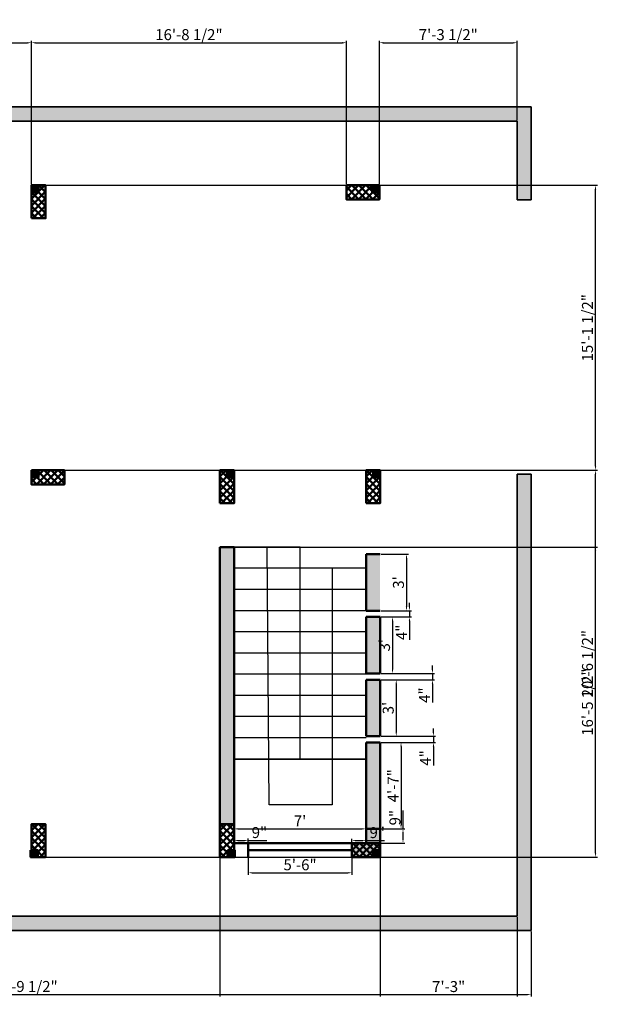
# Model space of a CAD drawing. Units: inches. Extents: x 1749 to 3550, y 1117 to 2383.
# Tile 9 of 15: x 2287 to 2660, y 1756 to 2383. Entities that reach past the tile are written whole.
import ezdxf

# ---------------------------------------------------------------- set-up
doc = ezdxf.new("R2010")
doc.units = ezdxf.units.IN
for name, color, linetype, lineweight in [('A-ANNO-DIMS', 2, 'Continuous', 18), ('A-COLS', 10, 'Continuous', 50), ('A-FLOR-STRS', 53, 'Continuous', 25), ('A-WALL', 7, 'Continuous', 50), ('A-WALL-PATT', 8, 'Continuous', 13), ('C-PROP', 8, 'Continuous', 35)]:
    doc.layers.add(name, color=color, linetype=linetype, lineweight=lineweight)
doc.styles.get("Standard").update_dxf_attribs({"font": 'arial.ttf'})
doc.dimstyles.new('ISO-25', dxfattribs={"dimtxt": 7, "dimasz": 2.5, "dimexe": 1.25, "dimexo": 0.625, "dimtad": 1, "dimdec": 1, "dimlunit": 3, "dimtxsty": 'Standard', "dimcen": 2.5, "dimadec": 0, "dimazin": 0, "dimtfac": 1, "dimtdec": 1, "dimtmove": 0, "dimatfit": 3, "dimfxl": 1, "dimarcsym": 0})

# ---------------------------------------------------------------- blocks, each defined once
blk = doc.blocks.new('*D149')
at = {"layer": 'A-ANNO-DIMS', "color": 0, "lineweight": -2, "ltscale": 0.5, "transparency": 16777216}
for p, q in [((2423.6, 1859.29), (2423.6, 1868.91)), ((2426.1, 1867.66), (2505.1, 1867.66)), ((2507.6, 1859.29), (2507.6, 1868.91))]:
    blk.add_line(p, q, dxfattribs=at)
at = {"layer": 'A-ANNO-DIMS', "color": 0, "ltscale": 0.5, "transparency": 16777216}
for points in [[(2426.1, 1868.08), (2426.1, 1867.24), (2423.6, 1867.66)], [(2505.1, 1868.08), (2505.1, 1867.24), (2507.6, 1867.66)]]:
    blk.add_solid(points, dxfattribs=at)
at = {"layer": 'Defpoints', "color": 0, "ltscale": 0.5, "transparency": 16777216}
for p in [(2507.6, 1867.66), (2423.6, 1858.66), (2507.6, 1858.66)]:
    blk.add_point(p, dxfattribs=at)
at = {"layer": 'A-ANNO-DIMS', "color": 0, "ltscale": 0.5, "transparency": 16777216, "insert": (2465.6, 1871.79), "char_height": 7, "attachment_point": 5}
blk.add_mtext("7'", dxfattribs=at)
blk = doc.blocks.new('*D143')
at = {"layer": 'A-ANNO-DIMS', "color": 0, "lineweight": -2, "ltscale": 0.5, "transparency": 16777216}
for p, q in [((2517.23, 2042.66), (2534.61, 2042.66)), ((2533.36, 2040.16), (2533.36, 2009.16)), ((2517.23, 2006.66), (2534.61, 2006.66))]:
    blk.add_line(p, q, dxfattribs=at)
at = {"layer": 'A-ANNO-DIMS', "color": 0, "ltscale": 0.5, "transparency": 16777216}
for points in [[(2532.94, 2040.16), (2533.78, 2040.16), (2533.36, 2042.66)], [(2532.94, 2009.16), (2533.78, 2009.16), (2533.36, 2006.66)]]:
    blk.add_solid(points, dxfattribs=at)
at = {"layer": 'Defpoints', "color": 0, "ltscale": 0.5, "transparency": 16777216}
for p in [(2516.6, 2042.66), (2516.6, 2006.66), (2533.36, 2006.66)]:
    blk.add_point(p, dxfattribs=at)
at = {"layer": 'A-ANNO-DIMS', "color": 0, "ltscale": 0.5, "transparency": 16777216, "insert": (2529.16, 2024.66), "char_height": 7, "attachment_point": 5, "rotation": 90}
blk.add_mtext("3'", dxfattribs=at)
blk = doc.blocks.new('*D144')
at = {"layer": 'A-ANNO-DIMS', "color": 0, "lineweight": -2, "ltscale": 0.5, "transparency": 16777216}
for p, q in [((2535.25, 2009.16), (2535.25, 2011.66)), ((2517.23, 2006.66), (2536.5, 2006.66)), ((2517.23, 2002.66), (2536.5, 2002.66)), ((2535.25, 2006.66), (2535.25, 2002.66)), ((2535.25, 2000.16), (2535.25, 1988.08))]:
    blk.add_line(p, q, dxfattribs=at)
at = {"layer": 'A-ANNO-DIMS', "color": 0, "ltscale": 0.5, "transparency": 16777216}
for points in [[(2534.83, 2009.16), (2535.66, 2009.16), (2535.25, 2006.66)], [(2534.83, 2000.16), (2535.66, 2000.16), (2535.25, 2002.66)]]:
    blk.add_solid(points, dxfattribs=at)
at = {"layer": 'Defpoints', "color": 0, "ltscale": 0.5, "transparency": 16777216}
for p in [(2516.6, 2006.66), (2516.6, 2002.66), (2535.25, 2002.66)]:
    blk.add_point(p, dxfattribs=at)
at = {"layer": 'A-ANNO-DIMS', "color": 0, "ltscale": 0.5, "transparency": 16777216, "insert": (2531.12, 1992.87), "char_height": 7, "attachment_point": 5, "rotation": 90}
blk.add_mtext('4"', dxfattribs=at)
blk = doc.blocks.new('*D145')
at = {"layer": 'A-ANNO-DIMS', "color": 0, "lineweight": -2, "ltscale": 0.5, "transparency": 16777216}
for p, q in [((2517.23, 2002.66), (2525.75, 2002.66)), ((2524.5, 2000.16), (2524.5, 1969.16)), ((2517.23, 1966.66), (2525.75, 1966.66))]:
    blk.add_line(p, q, dxfattribs=at)
at = {"layer": 'A-ANNO-DIMS', "color": 0, "ltscale": 0.5, "transparency": 16777216}
for points in [[(2524.08, 2000.16), (2524.91, 2000.16), (2524.5, 2002.66)], [(2524.08, 1969.16), (2524.91, 1969.16), (2524.5, 1966.66)]]:
    blk.add_solid(points, dxfattribs=at)
at = {"layer": 'Defpoints', "color": 0, "ltscale": 0.5, "transparency": 16777216}
for p in [(2516.6, 2002.66), (2516.6, 1966.66), (2524.5, 1966.66)]:
    blk.add_point(p, dxfattribs=at)
at = {"layer": 'A-ANNO-DIMS', "color": 0, "ltscale": 0.5, "transparency": 16777216, "insert": (2520.29, 1984.66), "char_height": 7, "attachment_point": 5, "rotation": 90}
blk.add_mtext("3'", dxfattribs=at)
blk = doc.blocks.new('*D146')
at = {"layer": 'A-ANNO-DIMS', "color": 0, "lineweight": -2, "ltscale": 0.5, "transparency": 16777216}
for p, q in [((2549.88, 1969.16), (2549.88, 1971.66)), ((2517.23, 1966.66), (2551.13, 1966.66)), ((2549.88, 1966.66), (2549.88, 1962.66)), ((2517.23, 1962.66), (2551.13, 1962.66)), ((2549.88, 1960.16), (2549.88, 1948.08))]:
    blk.add_line(p, q, dxfattribs=at)
at = {"layer": 'A-ANNO-DIMS', "color": 0, "ltscale": 0.5, "transparency": 16777216}
for points in [[(2549.46, 1969.16), (2550.3, 1969.16), (2549.88, 1966.66)], [(2549.46, 1960.16), (2550.3, 1960.16), (2549.88, 1962.66)]]:
    blk.add_solid(points, dxfattribs=at)
at = {"layer": 'Defpoints', "color": 0, "ltscale": 0.5, "transparency": 16777216}
for p in [(2516.6, 1966.66), (2516.6, 1962.66), (2549.88, 1962.66)]:
    blk.add_point(p, dxfattribs=at)
at = {"layer": 'A-ANNO-DIMS', "color": 0, "ltscale": 0.5, "transparency": 16777216, "insert": (2545.75, 1952.87), "char_height": 7, "attachment_point": 5, "rotation": 90}
blk.add_mtext('4"', dxfattribs=at)
blk = doc.blocks.new('*D147')
at = {"layer": 'A-ANNO-DIMS', "color": 0, "lineweight": -2, "ltscale": 0.5, "transparency": 16777216}
for p, q in [((2517.23, 1962.66), (2528.1, 1962.66)), ((2526.85, 1960.16), (2526.85, 1929.16)), ((2517.23, 1926.66), (2528.1, 1926.66))]:
    blk.add_line(p, q, dxfattribs=at)
at = {"layer": 'A-ANNO-DIMS', "color": 0, "ltscale": 0.5, "transparency": 16777216}
for points in [[(2526.43, 1960.16), (2527.26, 1960.16), (2526.85, 1962.66)], [(2526.43, 1929.16), (2527.26, 1929.16), (2526.85, 1926.66)]]:
    blk.add_solid(points, dxfattribs=at)
at = {"layer": 'Defpoints', "color": 0, "ltscale": 0.5, "transparency": 16777216}
for p in [(2516.6, 1962.66), (2516.6, 1926.66), (2526.85, 1926.66)]:
    blk.add_point(p, dxfattribs=at)
at = {"layer": 'A-ANNO-DIMS', "color": 0, "ltscale": 0.5, "transparency": 16777216, "insert": (2522.64, 1944.66), "char_height": 7, "attachment_point": 5, "rotation": 90}
blk.add_mtext("3'", dxfattribs=at)
blk = doc.blocks.new('*D148')
at = {"layer": 'A-ANNO-DIMS', "color": 0, "lineweight": -2, "ltscale": 0.5, "transparency": 16777216}
for p, q in [((2517.23, 1926.66), (2551.76, 1926.66)), ((2550.51, 1929.16), (2550.51, 1931.66)), ((2550.51, 1926.66), (2550.51, 1922.66)), ((2517.23, 1922.66), (2551.76, 1922.66)), ((2550.51, 1920.16), (2550.51, 1908.08))]:
    blk.add_line(p, q, dxfattribs=at)
at = {"layer": 'A-ANNO-DIMS', "color": 0, "ltscale": 0.5, "transparency": 16777216}
for points in [[(2550.09, 1929.16), (2550.93, 1929.16), (2550.51, 1926.66)], [(2550.09, 1920.16), (2550.93, 1920.16), (2550.51, 1922.66)]]:
    blk.add_solid(points, dxfattribs=at)
at = {"layer": 'Defpoints', "color": 0, "ltscale": 0.5, "transparency": 16777216}
for p in [(2516.6, 1926.66), (2516.6, 1922.66), (2550.51, 1922.66)]:
    blk.add_point(p, dxfattribs=at)
at = {"layer": 'A-ANNO-DIMS', "color": 0, "ltscale": 0.5, "transparency": 16777216, "insert": (2546.38, 1912.87), "char_height": 7, "attachment_point": 5, "rotation": 90}
blk.add_mtext('4"', dxfattribs=at)
blk = doc.blocks.new('*D138')
at = {"layer": 'A-ANNO-DIMS', "color": 0, "lineweight": -2, "ltscale": 0.5, "transparency": 16777216}
for p, q in [((2517.23, 1922.66), (2531.15, 1922.66)), ((2529.9, 1920.16), (2529.9, 1870.16)), ((2517.23, 1867.66), (2531.15, 1867.66))]:
    blk.add_line(p, q, dxfattribs=at)
at = {"layer": 'A-ANNO-DIMS', "color": 0, "ltscale": 0.5, "transparency": 16777216}
for points in [[(2529.48, 1920.16), (2530.31, 1920.16), (2529.9, 1922.66)], [(2529.48, 1870.16), (2530.31, 1870.16), (2529.9, 1867.66)]]:
    blk.add_solid(points, dxfattribs=at)
at = {"layer": 'Defpoints', "color": 0, "ltscale": 0.5, "transparency": 16777216}
for p in [(2516.6, 1922.66), (2516.6, 1867.66), (2529.9, 1867.66)]:
    blk.add_point(p, dxfattribs=at)
at = {"layer": 'A-ANNO-DIMS', "color": 0, "ltscale": 0.5, "transparency": 16777216, "insert": (2525.77, 1895.16), "char_height": 7, "attachment_point": 5, "rotation": 90}
blk.add_mtext('4\'-7"', dxfattribs=at)
blk = doc.blocks.new('*D139')
at = {"layer": 'A-ANNO-DIMS', "color": 0, "lineweight": -2, "ltscale": 0.5, "transparency": 16777216}
for p, q in [((2531.15, 1867.66), (2531.15, 1879.46)), ((2517.23, 1867.66), (2532.4, 1867.66)), ((2531.15, 1861.16), (2531.15, 1865.16)), ((2517.23, 1858.66), (2532.4, 1858.66))]:
    blk.add_line(p, q, dxfattribs=at)
at = {"layer": 'A-ANNO-DIMS', "color": 0, "ltscale": 0.5, "transparency": 16777216}
for points in [[(2530.73, 1865.16), (2531.56, 1865.16), (2531.15, 1867.66)], [(2530.73, 1861.16), (2531.56, 1861.16), (2531.15, 1858.66)]]:
    blk.add_solid(points, dxfattribs=at)
at = {"layer": 'Defpoints', "color": 0, "ltscale": 0.5, "transparency": 16777216}
for p in [(2516.6, 1867.66), (2531.15, 1867.66), (2516.6, 1858.66)]:
    blk.add_point(p, dxfattribs=at)
at = {"layer": 'A-ANNO-DIMS', "color": 0, "ltscale": 0.5, "transparency": 16777216, "insert": (2526.95, 1874.81), "char_height": 7, "attachment_point": 5, "rotation": 90}
blk.add_mtext('9"', dxfattribs=at)
blk = doc.blocks.new('*D140')
at = {"layer": 'A-ANNO-DIMS', "color": 0, "lineweight": -2, "ltscale": 0.5, "transparency": 16777216}
for p, q in [((2423.6, 1859.29), (2423.6, 1861.47)), ((2426.1, 1860.22), (2430.1, 1860.22)), ((2432.6, 1859.29), (2432.6, 1861.47)), ((2432.6, 1860.22), (2444.4, 1860.22))]:
    blk.add_line(p, q, dxfattribs=at)
at = {"layer": 'A-ANNO-DIMS', "color": 0, "ltscale": 0.5, "transparency": 16777216}
for points in [[(2426.1, 1860.63), (2426.1, 1859.8), (2423.6, 1860.22)], [(2430.1, 1860.63), (2430.1, 1859.8), (2432.6, 1860.22)]]:
    blk.add_solid(points, dxfattribs=at)
at = {"layer": 'Defpoints', "color": 0, "ltscale": 0.5, "transparency": 16777216}
for p in [(2423.6, 1858.66), (2432.6, 1860.22), (2432.6, 1858.66)]:
    blk.add_point(p, dxfattribs=at)
at = {"layer": 'A-ANNO-DIMS', "color": 0, "ltscale": 0.5, "transparency": 16777216, "insert": (2439.75, 1864.42), "char_height": 7, "attachment_point": 5}
blk.add_mtext('9"', dxfattribs=at)
blk = doc.blocks.new('*D141')
at = {"layer": 'A-ANNO-DIMS', "color": 0, "lineweight": -2, "ltscale": 0.5, "transparency": 16777216}
for p, q in [((2432.6, 1849.04), (2432.6, 1838.45)), ((2498.6, 1849.04), (2498.6, 1838.45)), ((2435.1, 1839.7), (2496.1, 1839.7))]:
    blk.add_line(p, q, dxfattribs=at)
at = {"layer": 'A-ANNO-DIMS', "color": 0, "ltscale": 0.5, "transparency": 16777216}
for points in [[(2435.1, 1840.12), (2435.1, 1839.29), (2432.6, 1839.7)], [(2496.1, 1840.12), (2496.1, 1839.29), (2498.6, 1839.7)]]:
    blk.add_solid(points, dxfattribs=at)
at = {"layer": 'Defpoints', "color": 0, "ltscale": 0.5, "transparency": 16777216}
for p in [(2432.6, 1849.66), (2498.6, 1849.66), (2498.6, 1839.7)]:
    blk.add_point(p, dxfattribs=at)
at = {"layer": 'A-ANNO-DIMS', "color": 0, "ltscale": 0.5, "transparency": 16777216, "insert": (2465.6, 1843.9), "char_height": 7, "attachment_point": 5}
blk.add_mtext('5\'-6"', dxfattribs=at)
blk = doc.blocks.new('*D142')
at = {"layer": 'A-ANNO-DIMS', "color": 0, "lineweight": -2, "ltscale": 0.5, "transparency": 16777216}
for p, q in [((2498.6, 1859.29), (2498.6, 1861.42)), ((2501.1, 1860.17), (2505.1, 1860.17)), ((2507.6, 1859.29), (2507.6, 1861.42)), ((2507.6, 1860.17), (2519.4, 1860.17))]:
    blk.add_line(p, q, dxfattribs=at)
at = {"layer": 'A-ANNO-DIMS', "color": 0, "ltscale": 0.5, "transparency": 16777216}
for points in [[(2501.1, 1860.59), (2501.1, 1859.75), (2498.6, 1860.17)], [(2505.1, 1860.59), (2505.1, 1859.75), (2507.6, 1860.17)]]:
    blk.add_solid(points, dxfattribs=at)
at = {"layer": 'Defpoints', "color": 0, "ltscale": 0.5, "transparency": 16777216}
for p in [(2498.6, 1858.66), (2507.6, 1860.17), (2507.6, 1858.66)]:
    blk.add_point(p, dxfattribs=at)
at = {"layer": 'A-ANNO-DIMS', "color": 0, "ltscale": 0.5, "transparency": 16777216, "insert": (2514.75, 1864.37), "char_height": 7, "attachment_point": 5}
blk.add_mtext('9"', dxfattribs=at)
blk = doc.blocks.new('*D157')
at = {"layer": 'A-ANNO-DIMS', "color": 0, "lineweight": -2, "ltscale": 0.5, "transparency": 16777216}
for p, q in [((1804.37, 1802.38), (1804.37, 1760.85)), ((2612.84, 1802.38), (2612.84, 1760.85)), ((1806.87, 1762.1), (2610.34, 1762.1))]:
    blk.add_line(p, q, dxfattribs=at)
at = {"layer": 'A-ANNO-DIMS', "color": 0, "ltscale": 0.5, "transparency": 16777216}
for points in [[(1806.87, 1762.52), (1806.87, 1761.69), (1804.37, 1762.1)], [(2610.34, 1762.52), (2610.34, 1761.69), (2612.84, 1762.1)]]:
    blk.add_solid(points, dxfattribs=at)
at = {"layer": 'Defpoints', "color": 0, "ltscale": 0.5, "transparency": 16777216}
for p in [(1804.37, 1803), (2612.84, 1803), (2612.84, 1762.1)]:
    blk.add_point(p, dxfattribs=at)
at = {"layer": 'A-ANNO-DIMS', "color": 0, "ltscale": 0.5, "transparency": 16777216, "insert": (2208.61, 1766.35), "char_height": 7, "attachment_point": 5}
blk.add_mtext('67\'-4 1/2"', dxfattribs=at)
blk = doc.blocks.new('*D164')
at = {"layer": 'A-ANNO-DIMS', "color": 0, "lineweight": -2, "ltscale": 0.5, "transparency": 16777216}
for p, q in [((2165.1, 2279.29), (2165.1, 2369.73)), ((2167.6, 2368.48), (2292.1, 2368.48)), ((2294.6, 2278.29), (2294.6, 2369.73))]:
    blk.add_line(p, q, dxfattribs=at)
at = {"layer": 'A-ANNO-DIMS', "color": 0, "ltscale": 0.5, "transparency": 16777216}
for points in [[(2167.6, 2368.9), (2167.6, 2368.06), (2165.1, 2368.48)], [(2292.1, 2368.9), (2292.1, 2368.06), (2294.6, 2368.48)]]:
    blk.add_solid(points, dxfattribs=at)
at = {"layer": 'Defpoints', "color": 0, "ltscale": 0.5, "transparency": 16777216}
for p in [(2294.6, 2368.48), (2165.1, 2278.66), (2294.6, 2277.66)]:
    blk.add_point(p, dxfattribs=at)
at = {"layer": 'A-ANNO-DIMS', "color": 0, "ltscale": 0.5, "transparency": 16777216, "insert": (2229.85, 2372.73), "char_height": 7, "attachment_point": 5}
blk.add_mtext('10\'-9 1/2"', dxfattribs=at)
blk = doc.blocks.new('*D165')
at = {"layer": 'A-ANNO-DIMS', "color": 0, "lineweight": -2, "ltscale": 0.5, "transparency": 16777216}
for p, q in [((2294.6, 2278.29), (2294.6, 2369.73)), ((2297.1, 2368.48), (2492.6, 2368.48)), ((2495.1, 2278.29), (2495.1, 2369.73))]:
    blk.add_line(p, q, dxfattribs=at)
at = {"layer": 'A-ANNO-DIMS', "color": 0, "ltscale": 0.5, "transparency": 16777216}
for points in [[(2297.1, 2368.9), (2297.1, 2368.06), (2294.6, 2368.48)], [(2492.6, 2368.9), (2492.6, 2368.06), (2495.1, 2368.48)]]:
    blk.add_solid(points, dxfattribs=at)
at = {"layer": 'Defpoints', "color": 0, "ltscale": 0.5, "transparency": 16777216}
for p in [(2495.1, 2368.48), (2294.6, 2277.66), (2495.1, 2277.66)]:
    blk.add_point(p, dxfattribs=at)
at = {"layer": 'A-ANNO-DIMS', "color": 0, "ltscale": 0.5, "transparency": 16777216, "insert": (2394.85, 2372.73), "char_height": 7, "attachment_point": 5}
blk.add_mtext('16\'-8 1/2"', dxfattribs=at)
blk = doc.blocks.new('*D166')
at = {"layer": 'A-ANNO-DIMS', "color": 0, "lineweight": -2, "ltscale": 0.5, "transparency": 16777216}
for p, q in [((2516.1, 2278.29), (2516.1, 2369.73)), ((2518.6, 2368.48), (2601.34, 2368.48)), ((2603.84, 2319.21), (2603.84, 2369.73))]:
    blk.add_line(p, q, dxfattribs=at)
at = {"layer": 'A-ANNO-DIMS', "color": 0, "ltscale": 0.5, "transparency": 16777216}
for points in [[(2518.6, 2368.9), (2518.6, 2368.06), (2516.1, 2368.48)], [(2601.34, 2368.9), (2601.34, 2368.06), (2603.84, 2368.48)]]:
    blk.add_solid(points, dxfattribs=at)
at = {"layer": 'Defpoints', "color": 0, "ltscale": 0.5, "transparency": 16777216}
for p in [(2603.84, 2368.48), (2603.84, 2318.58), (2516.1, 2277.66)]:
    blk.add_point(p, dxfattribs=at)
at = {"layer": 'A-ANNO-DIMS', "color": 0, "ltscale": 0.5, "transparency": 16777216, "insert": (2559.97, 2372.73), "char_height": 7, "attachment_point": 5}
blk.add_mtext('7\'-3 1/2"', dxfattribs=at)
blk = doc.blocks.new('*D167')
at = {"layer": 'A-ANNO-DIMS', "color": 0, "lineweight": -2, "ltscale": 0.5, "transparency": 16777216}
for p, q in [((2165.1, 1849.04), (2165.1, 1760.85)), ((2414.6, 1849.04), (2414.6, 1760.85)), ((2167.6, 1762.1), (2412.1, 1762.1))]:
    blk.add_line(p, q, dxfattribs=at)
at = {"layer": 'A-ANNO-DIMS', "color": 0, "ltscale": 0.5, "transparency": 16777216}
for points in [[(2167.6, 1762.52), (2167.6, 1761.69), (2165.1, 1762.1)], [(2412.1, 1762.52), (2412.1, 1761.69), (2414.6, 1762.1)]]:
    blk.add_solid(points, dxfattribs=at)
at = {"layer": 'Defpoints', "color": 0, "ltscale": 0.5, "transparency": 16777216}
for p in [(2165.1, 1849.66), (2414.6, 1849.66), (2414.6, 1762.1)]:
    blk.add_point(p, dxfattribs=at)
at = {"layer": 'A-ANNO-DIMS', "color": 0, "ltscale": 0.5, "transparency": 16777216, "insert": (2289.85, 1766.35), "char_height": 7, "attachment_point": 5}
blk.add_mtext('20\'-9 1/2"', dxfattribs=at)
blk = doc.blocks.new('*D168')
at = {"layer": 'A-ANNO-DIMS', "color": 0, "lineweight": -2, "ltscale": 0.5, "transparency": 16777216}
for p, q in [((2516.6, 1849.04), (2516.6, 1760.85)), ((2603.84, 1811.38), (2603.84, 1760.85)), ((2519.1, 1762.1), (2601.34, 1762.1))]:
    blk.add_line(p, q, dxfattribs=at)
at = {"layer": 'A-ANNO-DIMS', "color": 0, "ltscale": 0.5, "transparency": 16777216}
for points in [[(2519.1, 1762.52), (2519.1, 1761.69), (2516.6, 1762.1)], [(2601.34, 1762.52), (2601.34, 1761.69), (2603.84, 1762.1)]]:
    blk.add_solid(points, dxfattribs=at)
at = {"layer": 'Defpoints', "color": 0, "ltscale": 0.5, "transparency": 16777216}
for p in [(2516.6, 1849.66), (2603.84, 1812), (2603.84, 1762.1)]:
    blk.add_point(p, dxfattribs=at)
at = {"layer": 'A-ANNO-DIMS', "color": 0, "ltscale": 0.5, "transparency": 16777216, "insert": (2560.22, 1766.3), "char_height": 7, "attachment_point": 5}
blk.add_mtext('7\'-3"', dxfattribs=at)
blk = doc.blocks.new('*D169')
at = {"layer": 'A-ANNO-DIMS', "color": 0, "lineweight": -2, "ltscale": 0.5, "transparency": 16777216}
for p, q in [((2295.23, 2096.16), (2654.99, 2096.16)), ((2653.74, 1852.16), (2653.74, 2093.66)), ((2295.23, 1849.66), (2654.99, 1849.66))]:
    blk.add_line(p, q, dxfattribs=at)
at = {"layer": 'A-ANNO-DIMS', "color": 0, "ltscale": 0.5, "transparency": 16777216}
for points in [[(2653.33, 2093.66), (2654.16, 2093.66), (2653.74, 2096.16)], [(2653.33, 1852.16), (2654.16, 1852.16), (2653.74, 1849.66)]]:
    blk.add_solid(points, dxfattribs=at)
at = {"layer": 'Defpoints', "color": 0, "ltscale": 0.5, "transparency": 16777216}
for p in [(2294.6, 2096.16), (2653.74, 2096.16), (2294.6, 1849.66)]:
    blk.add_point(p, dxfattribs=at)
at = {"layer": 'A-ANNO-DIMS', "color": 0, "ltscale": 0.5, "transparency": 16777216, "insert": (2649.5, 1972.91), "char_height": 7, "attachment_point": 5, "rotation": 90}
blk.add_mtext('20\'-6 1/2"', dxfattribs=at)
blk = doc.blocks.new('*D170')
at = {"layer": 'A-ANNO-DIMS', "color": 0, "lineweight": -2, "ltscale": 0.5, "transparency": 16777216}
for p, q in [((2295.23, 2277.66), (2654.99, 2277.66)), ((2653.74, 2098.66), (2653.74, 2275.16)), ((2295.23, 2096.16), (2654.99, 2096.16))]:
    blk.add_line(p, q, dxfattribs=at)
at = {"layer": 'A-ANNO-DIMS', "color": 0, "ltscale": 0.5, "transparency": 16777216}
for points in [[(2653.33, 2275.16), (2654.16, 2275.16), (2653.74, 2277.66)], [(2653.33, 2098.66), (2654.16, 2098.66), (2653.74, 2096.16)]]:
    blk.add_solid(points, dxfattribs=at)
at = {"layer": 'Defpoints', "color": 0, "ltscale": 0.5, "transparency": 16777216}
for p in [(2294.6, 2277.66), (2653.74, 2277.66), (2294.6, 2096.16)]:
    blk.add_point(p, dxfattribs=at)
at = {"layer": 'A-ANNO-DIMS', "color": 0, "ltscale": 0.5, "transparency": 16777216, "insert": (2649.5, 2186.91), "char_height": 7, "attachment_point": 5, "rotation": 90}
blk.add_mtext('15\'-1 1/2"', dxfattribs=at)
blk = doc.blocks.new('*D171')
at = {"layer": 'A-ANNO-DIMS', "color": 0, "lineweight": -2, "ltscale": 0.5, "transparency": 16777216}
for p, q in [((2415.23, 2047.16), (2654.99, 2047.16)), ((2653.74, 1852.16), (2653.74, 2044.66)), ((2415.23, 1849.66), (2654.99, 1849.66))]:
    blk.add_line(p, q, dxfattribs=at)
at = {"layer": 'A-ANNO-DIMS', "color": 0, "ltscale": 0.5, "transparency": 16777216}
for points in [[(2653.33, 2044.66), (2654.16, 2044.66), (2653.74, 2047.16)], [(2653.33, 1852.16), (2654.16, 1852.16), (2653.74, 1849.66)]]:
    blk.add_solid(points, dxfattribs=at)
at = {"layer": 'Defpoints', "color": 0, "ltscale": 0.5, "transparency": 16777216}
for p in [(2414.6, 2047.16), (2653.74, 2047.16), (2414.6, 1849.66)]:
    blk.add_point(p, dxfattribs=at)
at = {"layer": 'A-ANNO-DIMS', "color": 0, "ltscale": 0.5, "transparency": 16777216, "insert": (2649.5, 1948.41), "char_height": 7, "attachment_point": 5, "rotation": 90}
blk.add_mtext('16\'-5 1/2"', dxfattribs=at)

msp = doc.modelspace()

# ---------------------------------------------------------------- hatches: boundary and pattern name
at = {"layer": 'A-COLS', "ltscale": 10}
h = msp.add_hatch(color=256, dxfattribs=at)
h.dxf.hatch_style = 1
h.paths.add_polyline_path([(2294.6, 2277.66), (2294.6, 2273.16), (2299.1, 2273.16), (2299.1, 2277.66)])
h = msp.add_hatch(dxfattribs=at)
h.set_pattern_fill('ANSI37', color=256, angle=90)
h.set_pattern_definition([(135, (3661.7103, 605.4172), (-2.245064, -2.245064), []), (225, (3661.7103, 605.4172), (2.245064, -2.245064), [])])
h.paths.add_polyline_path([(2303.6, 2277.66), (2294.6, 2277.66), (2294.6, 2256.66), (2303.6, 2256.66)])
h = msp.add_hatch(dxfattribs=at)
h.set_pattern_fill('ANSI37', color=256)
h.set_pattern_definition([(45, (843.86, 910.5555), (-2.245064, 2.245064), []), (135, (843.86, 910.5555), (-2.245064, -2.245064), [])])
h.paths.add_polyline_path([(2516.1, 2268.66), (2516.1, 2277.66), (2495.1, 2277.66), (2495.1, 2268.66)])
h = msp.add_hatch(color=256, dxfattribs=at)
h.dxf.hatch_style = 1
h.paths.add_polyline_path([(2511.6, 2277.66), (2511.6, 2273.16), (2516.1, 2273.16), (2516.1, 2277.66)])
h = msp.add_hatch(color=256, dxfattribs=at)
h.dxf.hatch_style = 1
h.paths.add_polyline_path([(2294.6, 2096.16), (2294.6, 2091.66), (2299.1, 2091.66), (2299.1, 2096.16)])
h = msp.add_hatch(dxfattribs=at)
h.set_pattern_fill('ANSI37', color=256)
h.set_pattern_definition([(45, (643.36, 729.0555), (-2.245064, 2.245064), []), (135, (643.36, 729.0555), (-2.245064, -2.245064), [])])
h.paths.add_polyline_path([(2315.6, 2087.16), (2315.6, 2096.16), (2294.6, 2096.16), (2294.6, 2087.16)])
h = msp.add_hatch(dxfattribs=at)
h.set_pattern_fill('ANSI37', color=256, angle=90)
h.set_pattern_definition([(135, (3781.7103, 423.9172), (-2.245064, -2.245064), []), (225, (3781.7103, 423.9172), (2.245064, -2.245064), [])])
h.paths.add_polyline_path([(2423.6, 2096.16), (2414.6, 2096.16), (2414.6, 2075.16), (2423.6, 2075.16)])
h = msp.add_hatch(color=256, dxfattribs=at)
h.dxf.hatch_style = 1
h.paths.add_polyline_path([(2419.1, 2096.16), (2419.1, 2091.66), (2423.6, 2091.66), (2423.6, 2096.16)])
h = msp.add_hatch(dxfattribs=at)
h.set_pattern_fill('ANSI37', color=256, angle=90)
h.set_pattern_definition([(135, (3874.7103, 423.9172), (-2.245064, -2.245064), []), (225, (3874.7103, 423.9172), (2.245064, -2.245064), [])])
h.paths.add_polyline_path([(2516.6, 2096.16), (2507.6, 2096.16), (2507.6, 2075.16), (2516.6, 2075.16)])
h = msp.add_hatch(color=256, dxfattribs=at)
h.dxf.hatch_style = 1
h.paths.add_polyline_path([(2512.1, 2096.16), (2512.1, 2091.66), (2516.6, 2091.66), (2516.6, 2096.16)])
h = msp.add_hatch(dxfattribs=at)
h.set_pattern_fill('ANSI37', color=256, angle=90)
h.set_pattern_definition([(135, (3661.7103, 198.4172), (-2.245064, -2.245064), []), (225, (3661.7103, 198.4172), (2.245064, -2.245064), [])])
h.paths.add_polyline_path([(2303.6, 1870.66), (2294.6, 1870.66), (2294.6, 1849.66), (2303.6, 1849.66)])
h = msp.add_hatch(dxfattribs=at)
h.set_pattern_fill('ANSI37', color=256, angle=90)
h.set_pattern_definition([(135, (3781.7103, 198.4172), (-2.245064, -2.245064), []), (225, (3781.7103, 198.4172), (2.245064, -2.245064), [])])
h.paths.add_polyline_path([(2423.6, 1870.66), (2414.6, 1870.66), (2414.6, 1849.66), (2423.6, 1849.66)])
h = msp.add_hatch(dxfattribs=at)
h.set_pattern_fill('ANSI37', color=256)
h.set_pattern_definition([(45, (844.36, 491.5555), (-2.245064, 2.245064), []), (135, (844.36, 491.5555), (-2.245064, -2.245064), [])])
h.paths.add_polyline_path([(2516.6, 1849.66), (2516.6, 1858.66), (2498.6, 1858.66), (2498.6, 1849.66)])
h = msp.add_hatch(color=256, dxfattribs=at)
h.dxf.hatch_style = 1
h.paths.add_polyline_path([(2294.1, 1854.16), (2294.1, 1849.66), (2298.6, 1849.66), (2298.6, 1854.16)])
h = msp.add_hatch(color=256, dxfattribs=at)
h.dxf.hatch_style = 1
h.paths.add_polyline_path([(2419.5, 1854.16), (2419.5, 1849.66), (2424, 1849.66), (2424, 1854.16)])
h = msp.add_hatch(color=256, dxfattribs=at)
h.dxf.hatch_style = 1
h.paths.add_polyline_path([(2512.1, 1854.16), (2512.1, 1849.66), (2516.6, 1849.66), (2516.6, 1854.16)])
at = {"layer": 'A-WALL-PATT', "ltscale": 0.5}
h = msp.add_hatch(color=256, dxfattribs=at)
h.dxf.hatch_style = 1
h.paths.add_polyline_path([(2612.84, 2327.58), (1804.37, 2327.58), (1804.37, 1803), (2612.84, 1803), (2612.84, 2093.66), (2603.84, 2093.66), (2603.84, 1812), (1813.37, 1812), (1813.37, 2318.58), (2603.84, 2318.58), (2603.84, 2268.45), (2612.84, 2268.45)])
h = msp.add_hatch(color=256, dxfattribs=at)
h.dxf.hatch_style = 1
h.paths.add_polyline_path([(2423.6, 2047.16), (2414.6, 2047.16), (2414.6, 1916.16), (2414.6, 1912.16), (2414.6, 1870.66), (2423.6, 1870.66)])
at = {"layer": 'A-WALL-PATT', "ltscale": 10}
h = msp.add_hatch(color=256, dxfattribs=at)
h.dxf.hatch_style = 1
h.paths.add_polyline_path([(2507.6, 2006.66), (2516.6, 2006.66), (2516.6, 2042.66), (2507.6, 2042.66)])
h.paths.add_polyline_path([(2516.6, 2002.66), (2507.6, 2002.66), (2507.6, 1966.66), (2516.6, 1966.66)])
h.paths.add_polyline_path([(2516.6, 1962.66), (2507.6, 1962.66), (2507.6, 1926.66), (2516.6, 1926.66)])
h = msp.add_hatch(color=256, dxfattribs=at)
h.dxf.hatch_style = 1
h.paths.add_polyline_path([(2507.6, 1867.66), (2516.6, 1867.66), (2516.6, 1922.66), (2507.6, 1922.66)])
h = msp.add_hatch(color=256, dxfattribs=at)
h.dxf.hatch_style = 1
h.paths.add_polyline_path([(2516.6, 1849.66), (2516.6, 1867.66), (2507.6, 1867.66), (2507.6, 1858.66), (2498.6, 1858.66), (2498.6, 1849.66)])

# ---------------------------------------------------------------- linework, layer by layer
at = {"layer": 'A-COLS', "ltscale": 10}
for points in [[(2294.6, 2277.66), (2299.1, 2277.66), (2299.1, 2273.16), (2294.6, 2273.16)], [(2294.6, 2256.66), (2294.6, 2277.66), (2303.6, 2277.66), (2303.6, 2256.66)], [(2495.1, 2277.66), (2516.1, 2277.66), (2516.1, 2268.66), (2495.1, 2268.66)], [(2511.6, 2277.66), (2516.1, 2277.66), (2516.1, 2273.16), (2511.6, 2273.16)], [(2294.6, 2096.16), (2299.1, 2096.16), (2299.1, 2091.66), (2294.6, 2091.66)], [(2294.6, 2096.16), (2315.6, 2096.16), (2315.6, 2087.16), (2294.6, 2087.16)], [(2414.6, 2075.16), (2414.6, 2096.16), (2423.6, 2096.16), (2423.6, 2075.16)], [(2419.1, 2096.16), (2423.6, 2096.16), (2423.6, 2091.66), (2419.1, 2091.66)], [(2507.6, 2075.16), (2507.6, 2096.16), (2516.6, 2096.16), (2516.6, 2075.16)], [(2512.1, 2096.16), (2516.6, 2096.16), (2516.6, 2091.66), (2512.1, 2091.66)], [(2294.6, 1849.66), (2294.6, 1870.66), (2303.6, 1870.66), (2303.6, 1849.66)], [(2414.6, 1849.66), (2414.6, 1870.66), (2423.6, 1870.66), (2423.6, 1849.66)], [(2498.6, 1858.66), (2516.6, 1858.66), (2516.6, 1849.66), (2498.6, 1849.66)], [(2294.1, 1854.16), (2298.6, 1854.16), (2298.6, 1849.66), (2294.1, 1849.66)], [(2419.5, 1854.16), (2424, 1854.16), (2424, 1849.66), (2419.5, 1849.66)], [(2512.1, 1854.16), (2516.6, 1854.16), (2516.6, 1849.66), (2512.1, 1849.66)]]:
    msp.add_lwpolyline(points, close=True, dxfattribs=at)
at = {"layer": 'A-FLOR-STRS', "ltscale": 0.5}
for p, q in [((2512.1, 2096.16), (2516.6, 2096.16)), ((2465.63, 2047.16), (2423.6, 2047.16)), ((2445.9, 1882.88), (2444.62, 2047.16)), ((2465.63, 2033.66), (2465.63, 2047.16)), ((2507.6, 2042.66), (2507.66, 2033.66)), ((2507.66, 2033.66), (2423.6, 2033.66)), ((2465.63, 1912.16), (2465.63, 2033.66)), ((2485.98, 2033.66), (2485.98, 1882.88)), ((2507.66, 2020.16), (2423.6, 2020.16)), ((2507.66, 2006.66), (2423.6, 2006.66)), ((2507.66, 1993.16), (2423.6, 1993.16)), ((2507.66, 1979.66), (2423.6, 1979.66)), ((2507.66, 1966.16), (2423.6, 1966.16)), ((2507.66, 1952.66), (2423.6, 1952.66)), ((2507.66, 1939.16), (2423.6, 1939.16)), ((2507.66, 1925.66), (2423.6, 1925.66)), ((2423.6, 1912.16), (2507.6, 1912.16)), ((2507.66, 1912.16), (2423.6, 1912.16)), ((2485.98, 1882.88), (2445.9, 1882.88))]:
    msp.add_line(p, q, dxfattribs=at)
at = {"layer": 'A-WALL', "ltscale": 0.2}
for p, q in [((2294.6, 2268.66), (2294.6, 2277.66)), ((2495.1, 2268.66), (2495.1, 2277.66)), ((2294.6, 2087.16), (2294.6, 2096.16)), ((2516.6, 2096.16), (2512.6, 2096.16)), ((2414.6, 2087.16), (2414.6, 2075.16)), ((2414.6, 2047.16), (2414.6, 1916.16)), ((2507.6, 2042.66), (2516.6, 2042.66)), ((2507.6, 2042.66), (2507.6, 2006.66)), ((2507.6, 2006.66), (2516.6, 2006.66)), ((2507.6, 2002.66), (2507.6, 1966.66)), ((2507.6, 2002.66), (2516.6, 2002.66)), ((2516.6, 2002.66), (2516.6, 1966.66)), ((2507.6, 1966.66), (2516.6, 1966.66)), ((2507.6, 1962.66), (2507.6, 1926.66)), ((2507.6, 1962.66), (2516.6, 1962.66)), ((2516.6, 1962.66), (2516.6, 1926.66)), ((2507.6, 1926.66), (2516.6, 1926.66)), ((2507.6, 1922.66), (2507.6, 1858.66)), ((2507.6, 1922.66), (2516.6, 1922.66)), ((2516.6, 1922.66), (2516.6, 1849.66)), ((2414.6, 1912.16), (2414.6, 1853.66)), ((2294.6, 1861.66), (2294.6, 1849.66)), ((2423.6, 1858.66), (2507.6, 1858.66)), ((2432.6, 1858.66), (2432.6, 1849.66)), ((2498.6, 1858.66), (2498.6, 1849.66)), ((2432.6, 1854.16), (2498.6, 1854.16)), ((2498.6, 1849.66), (2516.6, 1849.66))]:
    msp.add_line(p, q, dxfattribs=at)
at = {"layer": 'A-WALL', "ltscale": 0.5}
for p, q in [((2423.6, 2047.16), (2414.6, 2047.16)), ((2423.6, 2047.16), (2423.6, 1858.66)), ((2414.6, 1912.16), (2414.6, 1916.16))]:
    msp.add_line(p, q, dxfattribs=at)
at = {"layer": 'A-WALL', "ltscale": 10}
for p, q in [((2507.6, 1867.66), (2516.6, 1867.66)), ((2298.6, 1853.66), (2298.6, 1849.66)), ((2414.6, 1853.66), (2414.6, 1849.66))]:
    msp.add_line(p, q, dxfattribs=at)
at = {"layer": 'C-PROP', "ltscale": 0.5}
for p, q in [((1804.37, 2327.58), (2612.84, 2327.58)), ((2612.84, 2327.58), (2612.84, 2268.45)), ((1813.37, 2318.58), (2603.84, 2318.58)), ((2603.84, 2318.58), (2603.84, 2268.45)), ((2603.84, 2268.45), (2612.84, 2268.45)), ((2603.84, 2093.66), (2612.84, 2093.66)), ((2603.84, 1812), (2603.84, 2093.66)), ((2612.84, 1803), (2612.84, 2093.66)), ((2603.84, 1812), (1813.37, 1812)), ((2612.84, 1803), (1804.37, 1803))]:
    msp.add_line(p, q, dxfattribs=at)

# ---------------------------------------------------------------- dimensions: what is measured, and where the dimension line sits
at = {"layer": 'A-ANNO-DIMS', "ltscale": 0.5}
for base, p1, p2, override, picture, middle in [((2294.6, 2368.48), (2165.1, 2278.66), (2294.6, 2277.66), {"dimdec": 1, "dimlfac": 1, "dimrnd": 0, "dimzin": 1, "dimdsep": 46, "dimlunit": 4, "dimfrac": 2}, '*D164', (2229.85, 2372.73)), ((2495.1, 2368.48), (2294.6, 2277.66), (2495.1, 2277.66), {"dimdec": 1, "dimlfac": 1, "dimrnd": 0, "dimzin": 1, "dimdsep": 46, "dimlunit": 4, "dimfrac": 2}, '*D165', (2394.85, 2372.73)), ((2603.84, 2368.48), (2516.1, 2277.66), (2603.84, 2318.58), {"dimdec": 1, "dimlfac": 1, "dimrnd": 0, "dimzin": 1, "dimdsep": 46, "dimlunit": 4, "dimfrac": 2}, '*D166', (2559.97, 2372.73)), ((2507.6, 1867.66), (2423.6, 1858.66), (2507.6, 1858.66), {"dimclrd": 0, "dimclre": 0, "dimclrt": 0}, '*D149', (2465.6, 1871.79)), ((2432.6, 1860.22), (2423.6, 1858.66), (2432.6, 1858.66), {"dimclrd": 0, "dimclre": 0, "dimclrt": 0}, '*D140', (2439.75, 1864.42)), ((2507.6, 1860.17), (2498.6, 1858.66), (2507.6, 1858.66), {"dimclrd": 0, "dimclre": 0, "dimclrt": 0}, '*D142', (2514.75, 1864.37)), ((2414.6, 1762.1), (2165.1, 1849.66), (2414.6, 1849.66), {"dimdec": 1, "dimlfac": 1, "dimrnd": 0, "dimzin": 1, "dimdsep": 46, "dimlunit": 4, "dimfrac": 2}, '*D167', (2289.85, 1766.35)), ((2498.6, 1839.7), (2432.6, 1849.66), (2498.6, 1849.66), {"dimclrd": 0, "dimclre": 0, "dimclrt": 0}, '*D141', (2465.6, 1843.9)), ((2603.84, 1762.1), (2516.6, 1849.66), (2603.84, 1812), {"dimdec": 1, "dimlfac": 1, "dimrnd": 0, "dimzin": 1, "dimdsep": 46, "dimlunit": 4, "dimfrac": 2}, '*D168', (2560.22, 1766.3)), ((2612.84, 1762.1), (1804.37, 1803), (2612.84, 1803), {"dimdec": 1, "dimlfac": 1, "dimrnd": 0, "dimzin": 1, "dimdsep": 46, "dimlunit": 4, "dimfrac": 2}, '*D157', (2208.61, 1766.35))]:
    dim = msp.add_linear_dim(base=base, p1=p1, p2=p2, dimstyle='ISO-25', override=override, dxfattribs=at)
    dim.commit()
    dim.dimension.update_dxf_attribs({"geometry": picture, "text_midpoint": middle})
for base, p1, p2, override, picture, middle in [((2653.74, 2277.66), (2294.6, 2096.16), (2294.6, 2277.66), {"dimdec": 1, "dimlfac": 1, "dimrnd": 0, "dimzin": 1, "dimdsep": 46, "dimlunit": 4, "dimfrac": 2}, '*D170', (2649.5, 2186.91)), ((2653.74, 2096.16), (2294.6, 1849.66), (2294.6, 2096.16), {"dimdec": 1, "dimlfac": 1, "dimrnd": 0, "dimzin": 1, "dimdsep": 46, "dimlunit": 4, "dimfrac": 2}, '*D169', (2649.5, 1972.91)), ((2653.74, 2047.16), (2414.6, 1849.66), (2414.6, 2047.16), {"dimdec": 1, "dimlfac": 1, "dimrnd": 0, "dimzin": 1, "dimdsep": 46, "dimlunit": 4, "dimfrac": 2}, '*D171', (2649.5, 1948.41)), ((2533.36, 2006.66), (2516.6, 2042.66), (2516.6, 2006.66), {"dimclrd": 0, "dimclre": 0, "dimclrt": 0}, '*D143', (2529.16, 2024.66)), ((2535.25, 2002.66), (2516.6, 2006.66), (2516.6, 2002.66), {"dimclrd": 0, "dimclre": 0, "dimclrt": 0}, '*D144', (2531.12, 1992.87)), ((2524.5, 1966.66), (2516.6, 2002.66), (2516.6, 1966.66), {"dimclrd": 0, "dimclre": 0, "dimclrt": 0}, '*D145', (2520.29, 1984.66)), ((2549.88, 1962.66), (2516.6, 1966.66), (2516.6, 1962.66), {"dimclrd": 0, "dimclre": 0, "dimclrt": 0}, '*D146', (2545.75, 1952.87)), ((2526.85, 1926.66), (2516.6, 1962.66), (2516.6, 1926.66), {"dimclrd": 0, "dimclre": 0, "dimclrt": 0}, '*D147', (2522.64, 1944.66)), ((2550.51, 1922.66), (2516.6, 1926.66), (2516.6, 1922.66), {"dimclrd": 0, "dimclre": 0, "dimclrt": 0}, '*D148', (2546.38, 1912.87)), ((2529.9, 1867.66), (2516.6, 1922.66), (2516.6, 1867.66), {"dimclrd": 0, "dimclre": 0, "dimclrt": 0}, '*D138', (2525.77, 1895.16)), ((2531.15, 1867.66), (2516.6, 1858.66), (2516.6, 1867.66), {"dimclrd": 0, "dimclre": 0, "dimclrt": 0}, '*D139', (2526.95, 1874.81))]:
    dim = msp.add_linear_dim(base=base, p1=p1, p2=p2, angle=90, dimstyle='ISO-25', override=override, dxfattribs=at)
    dim.commit()
    dim.dimension.update_dxf_attribs({"geometry": picture, "text_midpoint": middle})

doc.saveas('drawing.dxf')
